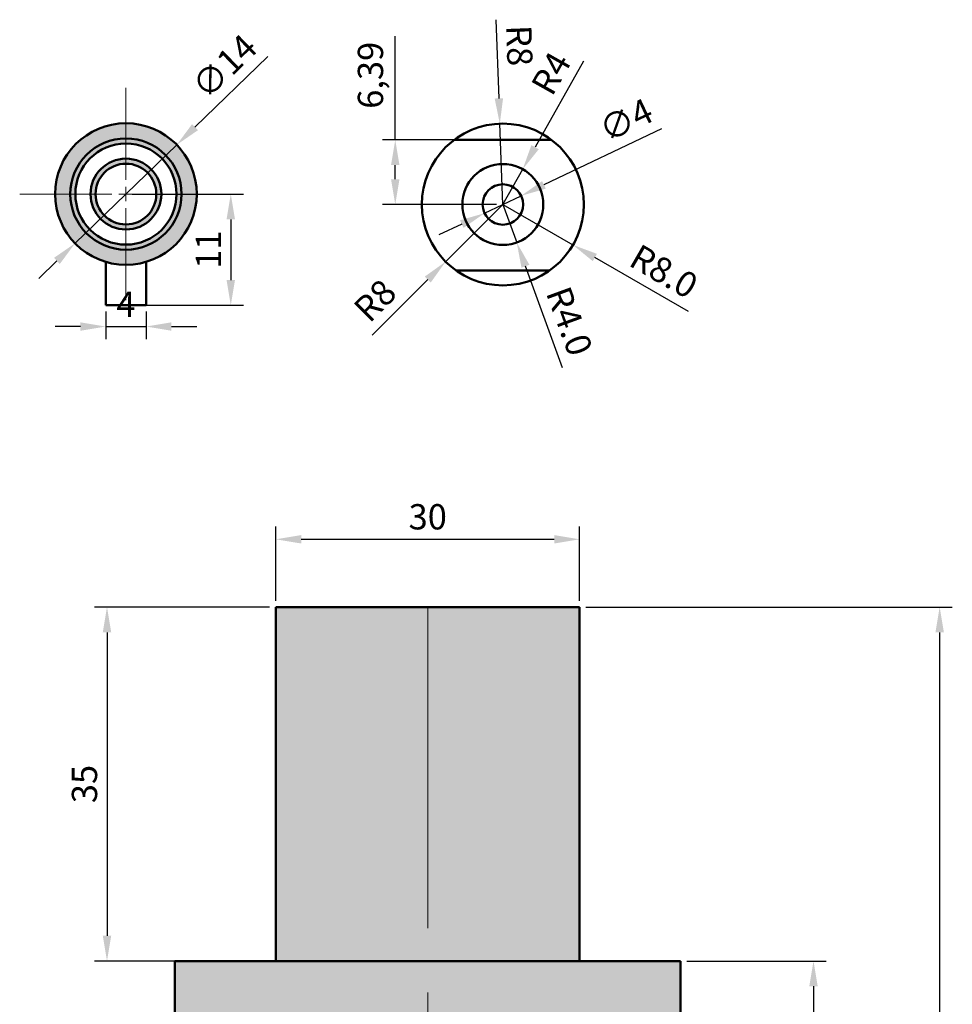
# Model space of a CAD drawing. Units: millimetres. Extents: x 1159 to 1466, y 1237 to 1440.
# Tile 3 of 6: x 1236 to 1329, y 1341 to 1438. Entities that reach past the tile are written whole.
import ezdxf

# ---------------------------------------------------------------- set-up
doc = ezdxf.new("R2010")
doc.units = ezdxf.units.MM
doc.linetypes.add('CENTER', pattern=[50.8, 31.75, -6.35, 6.35, -6.35])
for name, color, linetype, lineweight in [('M-CNTR', 1, 'CENTER', 18), ('M-DIMS', 2, 'Continuous', 25), ('M-HATC', 8, 'Continuous', 18), ('M-OUTL', 7, 'Continuous', 50)]:
    doc.layers.add(name, color=color, linetype=linetype, lineweight=lineweight)
doc.styles.get("Standard").update_dxf_attribs({"font": 'arial.ttf'})
doc.dimstyles.new('ISO-25', dxfattribs={"dimtxt": 2.5, "dimasz": 2.5, "dimexe": 1.25, "dimexo": 0.625, "dimtad": 1, "dimtxsty": 'Standard', "dimcen": 2.5, "dimadec": 0, "dimazin": 0, "dimtfac": 1, "dimtmove": 0, "dimatfit": 3, "dimfxl": 1, "dimarcsym": 0})

# ---------------------------------------------------------------- blocks, each defined once
blk = doc.blocks.new('*U1')
at = {"layer": 'M-CNTR', "color": 0, "transparency": 16777216}
for p, q in [((0, 1.4), (0, 10.5)), ((-10.5, 0), (-1.4, 0)), ((1.4, 0), (10.5, 0)), ((0, -10.5), (0, -1.4))]:
    blk.add_line(p, q, dxfattribs=at)
at = {"layer": 'M-CNTR', "color": 0, "linetype": 'Continuous', "transparency": 16777216}
for p, q in [((-0.7, 0), (0.7, 0)), ((0, -0.7), (0, 0.7))]:
    blk.add_line(p, q, dxfattribs=at)
blk = doc.blocks.new('*D3')
at = {"layer": 'Defpoints', "color": 0, "transparency": 16777216}
for p in [(1246.833, 1421.099), (1246.833, 1410.099), (1257.194, 1410.099)]:
    blk.add_point(p, dxfattribs=at)
at = {"layer": 'M-DIMS', "color": 0, "lineweight": -2, "transparency": 16777216}
for p, q in [((1247.458, 1421.099), (1258.444, 1421.099)), ((1257.194, 1418.599), (1257.194, 1412.599)), ((1247.458, 1410.099), (1258.444, 1410.099))]:
    blk.add_line(p, q, dxfattribs=at)
at = {"layer": 'M-DIMS', "color": 0, "transparency": 16777216}
for points in [[(1256.778, 1418.599), (1257.611, 1418.599), (1257.194, 1421.099)], [(1256.778, 1412.599), (1257.611, 1412.599), (1257.194, 1410.099)]]:
    blk.add_solid(points, dxfattribs=at)
at = {"layer": 'M-DIMS', "color": 0, "transparency": 16777216, "insert": (1255.314, 1415.599), "char_height": 2.5, "attachment_point": 5, "rotation": 90}
blk.add_mtext('11', dxfattribs=at)
blk = doc.blocks.new('*D4')
at = {"layer": 'Defpoints', "color": 0, "transparency": 16777216}
for p in [(1251.86, 1425.97), (1241.805, 1416.228)]:
    blk.add_point(p, dxfattribs=at)
at = {"layer": 'M-DIMS', "color": 0, "lineweight": -2, "transparency": 16777216}
for p, q in [((1260.867, 1434.697), (1253.656, 1427.71)), ((1241.805, 1416.228), (1251.86, 1425.97)), ((1240.01, 1414.489), (1238.215, 1412.749))]:
    blk.add_line(p, q, dxfattribs=at)
at = {"layer": 'M-DIMS', "color": 0, "transparency": 16777216}
for points in [[(1253.366, 1428.009), (1253.946, 1427.411), (1251.86, 1425.97)], [(1239.72, 1414.788), (1240.3, 1414.19), (1241.805, 1416.228)]]:
    blk.add_solid(points, dxfattribs=at)
at = {"layer": 'M-DIMS', "color": 0, "transparency": 16777216, "insert": (1256.787, 1433.489), "char_height": 2.5, "attachment_point": 5, "rotation": 44.0947}
blk.add_mtext('∅14', dxfattribs=at)
blk = doc.blocks.new('*D5')
at = {"layer": 'Defpoints', "color": 0, "transparency": 16777216}
for p in [(1273.452, 1426.462), (1284.087, 1426.462), (1284.087, 1420.067)]:
    blk.add_point(p, dxfattribs=at)
at = {"layer": 'M-DIMS', "color": 0, "lineweight": -2, "transparency": 16777216}
for p, q in [((1273.452, 1426.462), (1273.452, 1436.724)), ((1283.462, 1426.462), (1272.202, 1426.462)), ((1273.452, 1422.567), (1273.452, 1423.962)), ((1283.462, 1420.067), (1272.202, 1420.067))]:
    blk.add_line(p, q, dxfattribs=at)
at = {"layer": 'M-DIMS', "color": 0, "transparency": 16777216}
for points in [[(1273.036, 1423.962), (1273.869, 1423.962), (1273.452, 1426.462)], [(1273.036, 1422.567), (1273.869, 1422.567), (1273.452, 1420.067)]]:
    blk.add_solid(points, dxfattribs=at)
at = {"layer": 'M-DIMS', "color": 0, "transparency": 16777216, "insert": (1271.325, 1432.843), "char_height": 2.5, "attachment_point": 5, "rotation": 90}
blk.add_mtext('6,39', dxfattribs=at)
blk = doc.blocks.new('*D6')
at = {"layer": 'Defpoints', "color": 0, "transparency": 16777216}
for p in [(1285.892, 1420.928), (1282.282, 1419.206)]:
    blk.add_point(p, dxfattribs=at)
at = {"layer": 'M-DIMS', "color": 0, "lineweight": -2, "transparency": 16777216}
for p, q in [((1299.765, 1427.543), (1288.149, 1422.004)), ((1282.282, 1419.206), (1285.892, 1420.928)), ((1280.025, 1418.13), (1277.769, 1417.054))]:
    blk.add_line(p, q, dxfattribs=at)
at = {"layer": 'M-DIMS', "color": 0, "transparency": 16777216}
for points in [[(1287.969, 1422.38), (1288.328, 1421.628), (1285.892, 1420.928)], [(1279.846, 1418.506), (1280.204, 1417.754), (1282.282, 1419.206)]]:
    blk.add_solid(points, dxfattribs=at)
at = {"layer": 'M-DIMS', "color": 0, "transparency": 16777216, "insert": (1296.39, 1428.118), "char_height": 2.5, "attachment_point": 5, "rotation": 25.49518}
blk.add_mtext('∅4', dxfattribs=at)
blk = doc.blocks.new('*D7')
at = {"layer": 'Defpoints', "color": 0, "transparency": 16777216}
for p in [(1286.047, 1423.554), (1284.087, 1420.067)]:
    blk.add_point(p, dxfattribs=at)
at = {"layer": 'M-DIMS', "color": 0, "lineweight": -2, "transparency": 16777216}
for p, q in [((1292.064, 1434.254), (1287.273, 1425.733)), ((1284.087, 1420.067), (1286.047, 1423.554))]:
    blk.add_line(p, q, dxfattribs=at)
at = {"layer": 'M-DIMS', "color": 0, "transparency": 16777216}
blk.add_solid([(1286.909, 1425.937), (1287.636, 1425.529), (1286.047, 1423.554)], dxfattribs=at)
at = {"layer": 'M-DIMS', "color": 0, "transparency": 16777216, "insert": (1289.138, 1432.875), "char_height": 2.5, "attachment_point": 5, "rotation": 60.65232}
blk.add_mtext('R4', dxfattribs=at)
blk = doc.blocks.new('*D8')
at = {"layer": 'Defpoints', "color": 0, "transparency": 16777216}
for p in [(1283.788, 1428.061), (1284.087, 1420.067)]:
    blk.add_point(p, dxfattribs=at)
at = {"layer": 'M-DIMS', "color": 0, "lineweight": -2, "transparency": 16777216}
for p, q in [((1283.404, 1438.341), (1283.695, 1430.56)), ((1284.087, 1420.067), (1283.788, 1428.061))]:
    blk.add_line(p, q, dxfattribs=at)
at = {"layer": 'M-DIMS', "color": 0, "transparency": 16777216}
blk.add_solid([(1284.111, 1430.575), (1283.278, 1430.544), (1283.788, 1428.061)], dxfattribs=at)
at = {"layer": 'M-DIMS', "color": 0, "transparency": 16777216, "insert": (1285.403, 1435.77), "char_height": 2.5, "attachment_point": 5, "rotation": 272.1397}
blk.add_mtext('R8', dxfattribs=at)
blk = doc.blocks.new('*D17')
at = {"layer": 'Defpoints', "color": 0, "transparency": 16777216}
for p in [(1291.662, 1380.26), (1286.662, 1271.159), (1327.261, 1271.159)]:
    blk.add_point(p, dxfattribs=at)
at = {"layer": 'M-DIMS', "color": 0, "lineweight": -2, "transparency": 16777216}
for p, q in [((1292.287, 1380.26), (1328.511, 1380.26)), ((1327.261, 1377.76), (1327.261, 1273.659)), ((1287.287, 1271.159), (1328.511, 1271.159))]:
    blk.add_line(p, q, dxfattribs=at)
at = {"layer": 'M-DIMS', "color": 0, "transparency": 16777216}
for points in [[(1326.844, 1377.76), (1327.678, 1377.76), (1327.261, 1380.26)], [(1326.844, 1273.659), (1327.678, 1273.659), (1327.261, 1271.159)]]:
    blk.add_solid(points, dxfattribs=at)
at = {"layer": 'M-DIMS', "color": 0, "transparency": 16777216, "insert": (1325.134, 1325.71), "char_height": 2.5, "attachment_point": 5, "rotation": 90}
blk.add_mtext('109,1', dxfattribs=at)
blk = doc.blocks.new('*D18')
at = {"layer": 'Defpoints', "color": 0, "transparency": 16777216}
for p in [(1301.662, 1345.26), (1300.162, 1322.76), (1314.79, 1322.76)]:
    blk.add_point(p, dxfattribs=at)
at = {"layer": 'M-DIMS', "color": 0, "lineweight": -2, "transparency": 16777216}
for p, q in [((1302.287, 1345.26), (1316.04, 1345.26)), ((1314.79, 1342.76), (1314.79, 1325.26)), ((1300.787, 1322.76), (1316.04, 1322.76))]:
    blk.add_line(p, q, dxfattribs=at)
at = {"layer": 'M-DIMS', "color": 0, "transparency": 16777216}
for points in [[(1314.373, 1342.76), (1315.207, 1342.76), (1314.79, 1345.26)], [(1314.373, 1325.26), (1315.207, 1325.26), (1314.79, 1322.76)]]:
    blk.add_solid(points, dxfattribs=at)
at = {"layer": 'M-DIMS', "color": 0, "transparency": 16777216, "insert": (1312.663, 1334.01), "char_height": 2.5, "attachment_point": 5, "rotation": 90}
blk.add_mtext('22,5', dxfattribs=at)
blk = doc.blocks.new('*D29')
at = {"layer": 'Defpoints', "color": 0, "transparency": 16777216}
for p in [(1291.662, 1386.96), (1261.662, 1380.26), (1291.662, 1380.26)]:
    blk.add_point(p, dxfattribs=at)
at = {"layer": 'M-DIMS', "color": 0, "lineweight": -2, "transparency": 16777216}
for p, q in [((1261.662, 1380.885), (1261.662, 1388.21)), ((1291.662, 1380.885), (1291.662, 1388.21)), ((1264.162, 1386.96), (1289.162, 1386.96))]:
    blk.add_line(p, q, dxfattribs=at)
at = {"layer": 'M-DIMS', "color": 0, "transparency": 16777216}
for points in [[(1264.162, 1387.377), (1264.162, 1386.544), (1261.662, 1386.96)], [(1289.162, 1387.377), (1289.162, 1386.544), (1291.662, 1386.96)]]:
    blk.add_solid(points, dxfattribs=at)
at = {"layer": 'M-DIMS', "color": 0, "transparency": 16777216, "insert": (1276.662, 1388.863), "char_height": 2.5, "attachment_point": 5}
blk.add_mtext('30', dxfattribs=at)
blk = doc.blocks.new('*D33')
at = {"layer": 'Defpoints', "color": 0, "transparency": 16777216}
for p in [(1261.662, 1380.26), (1244.962, 1345.26), (1261.662, 1345.26)]:
    blk.add_point(p, dxfattribs=at)
at = {"layer": 'M-DIMS', "color": 0, "lineweight": -2, "transparency": 16777216}
for p, q in [((1261.037, 1380.26), (1243.712, 1380.26)), ((1244.962, 1377.76), (1244.962, 1347.76)), ((1261.037, 1345.26), (1243.712, 1345.26))]:
    blk.add_line(p, q, dxfattribs=at)
at = {"layer": 'M-DIMS', "color": 0, "transparency": 16777216}
for points in [[(1244.545, 1377.76), (1245.378, 1377.76), (1244.962, 1380.26)], [(1244.545, 1347.76), (1245.378, 1347.76), (1244.962, 1345.26)]]:
    blk.add_solid(points, dxfattribs=at)
at = {"layer": 'M-DIMS', "color": 0, "transparency": 16777216, "insert": (1243.059, 1362.76), "char_height": 2.5, "attachment_point": 5, "rotation": 90}
blk.add_mtext('35', dxfattribs=at)
blk = doc.blocks.new('*D41')
at = {"layer": 'Defpoints', "color": 0, "transparency": 16777216}
for p in [(1244.833, 1410.099), (1248.833, 1410.099), (1248.833, 1407.999)]:
    blk.add_point(p, dxfattribs=at)
at = {"layer": 'M-DIMS', "color": 0, "lineweight": -2, "transparency": 16777216}
for p, q in [((1244.833, 1409.474), (1244.833, 1406.749)), ((1248.833, 1409.474), (1248.833, 1406.749)), ((1242.333, 1407.999), (1239.833, 1407.999)), ((1244.833, 1407.999), (1248.833, 1407.999)), ((1251.333, 1407.999), (1253.833, 1407.999))]:
    blk.add_line(p, q, dxfattribs=at)
at = {"layer": 'M-DIMS', "color": 0, "transparency": 16777216}
for points in [[(1242.333, 1408.416), (1242.333, 1407.583), (1244.833, 1407.999)], [(1251.333, 1408.416), (1251.333, 1407.583), (1248.833, 1407.999)]]:
    blk.add_solid(points, dxfattribs=at)
at = {"layer": 'M-DIMS', "color": 0, "transparency": 16777216, "insert": (1246.833, 1409.874), "char_height": 2.5, "attachment_point": 5}
blk.add_mtext('4', dxfattribs=at)
blk = doc.blocks.new('*D53')
at = {"layer": 'Defpoints', "color": 0, "transparency": 16777216}
for p in [(1284.087, 1420.067), (1278.43, 1414.41)]:
    blk.add_point(p, dxfattribs=at)
at = {"layer": 'M-DIMS', "color": 0, "lineweight": -2, "transparency": 16777216}
for p, q in [((1284.087, 1420.067), (1278.43, 1414.41)), ((1271.156, 1407.136), (1276.662, 1412.642))]:
    blk.add_line(p, q, dxfattribs=at)
at = {"layer": 'M-DIMS', "color": 0, "transparency": 16777216}
blk.add_solid([(1276.368, 1412.937), (1276.957, 1412.348), (1278.43, 1414.41)], dxfattribs=at)
at = {"layer": 'M-DIMS', "color": 0, "transparency": 16777216, "insert": (1271.681, 1410.35), "char_height": 2.5, "attachment_point": 5, "rotation": 45.00022}
blk.add_mtext('R8', dxfattribs=at)
blk = doc.blocks.new('*D92')
at = {"layer": 'Defpoints', "color": 0, "transparency": 16777216}
for p in [(1284.087, 1420.067), (1291.018, 1416.071)]:
    blk.add_point(p, dxfattribs=at)
at = {"layer": 'M-DIMS', "color": 0, "lineweight": -2, "transparency": 16777216}
for p, q in [((1284.087, 1420.067), (1291.018, 1416.071)), ((1302.441, 1409.486), (1293.184, 1414.823))]:
    blk.add_line(p, q, dxfattribs=at)
at = {"layer": 'M-DIMS', "color": 0, "transparency": 16777216}
blk.add_solid([(1293.392, 1415.184), (1292.975, 1414.462), (1291.018, 1416.071)], dxfattribs=at)
at = {"layer": 'M-DIMS', "color": 0, "transparency": 16777216, "insert": (1299.845, 1413.177), "char_height": 2.5, "attachment_point": 5, "rotation": 330.03652}
blk.add_mtext('R8.0', dxfattribs=at)
blk = doc.blocks.new('*D93')
at = {"layer": 'Defpoints', "color": 0, "transparency": 16777216}
for p in [(1284.087, 1420.067), (1285.46, 1416.31)]:
    blk.add_point(p, dxfattribs=at)
at = {"layer": 'M-DIMS', "color": 0, "lineweight": -2, "transparency": 16777216}
for p, q in [((1284.087, 1420.067), (1285.46, 1416.31)), ((1289.986, 1403.926), (1286.318, 1413.962))]:
    blk.add_line(p, q, dxfattribs=at)
at = {"layer": 'M-DIMS', "color": 0, "transparency": 16777216}
blk.add_solid([(1286.71, 1414.105), (1285.927, 1413.819), (1285.46, 1416.31)], dxfattribs=at)
at = {"layer": 'M-DIMS', "color": 0, "transparency": 16777216, "insert": (1290.367, 1408.422), "char_height": 2.5, "attachment_point": 5, "rotation": 290.07659}
blk.add_mtext('R4.0', dxfattribs=at)

msp = doc.modelspace()

# ---------------------------------------------------------------- hatches: boundary and pattern name
at = {"layer": 'M-HATC'}
h = msp.add_hatch(color=256, dxfattribs=at)
h.set_gradient(color1=(19, 103, 52))
h.paths.add_polyline_path([(1239.8328, 1421.0994), (1241.3328, 1421.0994, -0.4142136), (1246.8328, 1426.5994), (1246.8328, 1428.0994, 0.4142136)])
h.paths.add_polyline_path([(1246.8328, 1428.0994), (1246.8328, 1426.5994, -0.4142136), (1252.3328, 1421.0994), (1253.8328, 1421.0994, 0.4142136)])
h.paths.add_polyline_path([(1246.8328, 1415.5994), (1246.8328, 1414.0994, 0.4142136), (1253.8328, 1421.0994), (1252.3328, 1421.0994, -0.4142136)])
h.paths.add_polyline_path([(1246.8328, 1414.0994), (1246.8328, 1415.5994, -0.4142136), (1241.3328, 1421.0994), (1239.8328, 1421.0994, 0.4142136)])
h = msp.add_hatch(color=256, dxfattribs=at)
h.set_gradient(color1=(205, 32, 39))
h.paths.add_polyline_path([(1246.8328, 1426.0994), (1246.8328, 1426.5994, 0.4142136), (1241.3328, 1421.0994), (1241.8328, 1421.0994, -0.4142136)])
h.paths.add_polyline_path([(1251.8328, 1421.0994), (1252.3328, 1421.0994, 0.4142136), (1246.8328, 1426.5994), (1246.8328, 1426.0994, -0.4142136)])
h.paths.add_polyline_path([(1246.8328, 1416.0994), (1246.8328, 1415.5994, 0.4142136), (1252.3328, 1421.0994), (1251.8328, 1421.0994, -0.4142136)])
h.paths.add_polyline_path([(1241.8328, 1421.0994), (1241.3328, 1421.0994, 0.4142136), (1246.8328, 1415.5994), (1246.8328, 1416.0994, -0.4142136)])
h = msp.add_hatch(color=256, dxfattribs=at)
h.set_gradient(color2=(0, 0, 255))
h.paths.add_polyline_path([(1246.8328, 1424.0994), (1246.8328, 1424.5994, 0.4142136), (1243.3328, 1421.0994), (1243.8328, 1421.0994, -0.4142136)])
h.paths.add_polyline_path([(1249.8328, 1421.0994), (1250.3328, 1421.0994, 0.4142136), (1246.8328, 1424.5994), (1246.8328, 1424.0994, -0.4142136)])
h.paths.add_polyline_path([(1250.3328, 1421.0994), (1249.8328, 1421.0994, -0.4142136), (1246.8328, 1418.0994), (1246.8328, 1417.5994, 0.4142136)])
h.paths.add_polyline_path([(1243.8328, 1421.0994), (1243.3328, 1421.0994, 0.4142136), (1246.8328, 1417.5994), (1246.8328, 1418.0994, -0.4142136)])
h = msp.add_hatch(color=256, dxfattribs=at)
h.set_gradient(color1=(100, 33, 101))
h.paths.add_polyline_path([(1276.6615, 1380.2603), (1261.6615, 1380.2603), (1261.6615, 1345.2603), (1276.6615, 1345.2603)])
h.paths.add_polyline_path([(1291.6615, 1380.2603), (1276.6615, 1380.2603), (1276.6615, 1345.2603), (1291.6615, 1345.2603)])
h = msp.add_hatch(color=256, dxfattribs=at)
h.set_gradient(color1=(237, 31, 36), color2=(248, 215, 49))
h.paths.add_polyline_path([(1276.6615, 1345.2603), (1261.6615, 1345.2603), (1251.6615, 1345.2603), (1251.6615, 1322.7603), (1254.6615, 1322.7603), (1276.6615, 1322.7603)])
h.paths.add_polyline_path([(1301.6615, 1345.2603), (1291.6615, 1345.2603), (1276.6615, 1345.2603), (1276.6615, 1322.7603), (1298.6615, 1322.7603), (1301.6615, 1322.7603)])

# ---------------------------------------------------------------- linework, layer by layer
at = {"layer": 'M-CNTR'}
msp.add_line((1276.6615, 1380.2603), (1276.6615, 1271.159), dxfattribs=at)
at = {"layer": 'M-OUTL'}
for p, q in [((1279.2799, 1426.4617), (1288.8939, 1426.4617)), ((1244.8328, 1414.3912), (1244.8328, 1410.0994)), ((1248.8328, 1410.0994), (1248.8328, 1414.3912)), ((1288.6931, 1413.5261), (1279.4807, 1413.5261)), ((1246.8328, 1410.0994), (1244.8328, 1410.0994)), ((1246.8328, 1410.0994), (1248.8328, 1410.0994)), ((1261.6615, 1380.2603), (1291.6615, 1380.2603)), ((1261.6615, 1345.2603), (1261.6615, 1380.2603)), ((1291.6615, 1380.2603), (1291.6615, 1345.2603)), ((1261.6615, 1345.2603), (1251.6615, 1345.2603)), ((1251.6615, 1345.2603), (1251.6615, 1322.7603)), ((1291.6615, 1345.2603), (1261.6615, 1345.2603)), ((1301.6615, 1345.2603), (1291.6615, 1345.2603)), ((1301.6615, 1322.7603), (1301.6615, 1345.2603))]:
    msp.add_line(p, q, dxfattribs=at)
for centre, radius in [((1246.8328, 1421.0994), 7), ((1284.0869, 1420.0669), 8), ((1246.8328, 1421.0994), 5.5), ((1246.8328, 1421.0994), 5), ((1246.8328, 1421.0994), 3.5), ((1246.8328, 1421.0994), 3), ((1284.0869, 1420.0669), 4), ((1284.0869, 1420.0669), 2)]:
    msp.add_circle(centre, radius, dxfattribs=at)

# ---------------------------------------------------------------- block references
at = {"layer": 'M-CNTR'}
msp.add_blockref('*U1', (1246.8328, 1421.0994), dxfattribs=at)

# ---------------------------------------------------------------- dimensions: what is measured, and where the dimension line sits
at = {"layer": 'M-DIMS'}
for mpoint, override, picture, middle in [((1283.7882, 1428.0614), {"dimclrd": 0, "dimclre": 0, "dimclrt": 0}, '*D8', (1285.4029, 1435.7703)), ((1278.4301, 1414.4101), {"dimdec": 0, "dimlfac": 1, "dimrnd": 0, "dimzin": 0, "dimdsep": 46, "dimlunit": 2}, '*D53', (1271.681, 1410.35)), ((1291.0176, 1416.0714), {"dimdec": 1, "dimlfac": 1, "dimrnd": 0, "dimzin": 0, "dimdsep": 46, "dimlunit": 2}, '*D92', (1299.8448, 1413.1773)), ((1285.46, 1416.31), {"dimdec": 1, "dimlfac": 1, "dimrnd": 0, "dimzin": 0, "dimdsep": 46, "dimlunit": 2}, '*D93', (1290.3672, 1408.4225))]:
    dim = msp.add_radius_dim(center=(1284.0869, 1420.0669), mpoint=mpoint, dimstyle='ISO-25', override=override, dxfattribs=at)
    dim.commit()
    dim.dimension.update_dxf_attribs({"geometry": picture, "text_midpoint": middle})
dim = msp.add_diameter_dim_2p(p1=(1241.8055, 1416.2284), p2=(1251.8602, 1425.9703), dimstyle='ISO-25', override={"dimclrd": 0, "dimclre": 0, "dimclrt": 0}, dxfattribs=at)
dim.commit()
dim.dimension.update_dxf_attribs({"geometry": '*D4', "text_midpoint": (1256.7873, 1433.489)})
for base, p1, p2, override, picture, middle in [((1273.4525, 1426.4617), (1284.0869, 1420.0669), (1284.0869, 1426.4617), {"dimclrd": 0, "dimclre": 0, "dimclrt": 0}, '*D5', (1271.3251, 1432.843)), ((1257.1943, 1410.0994), (1246.8328, 1421.0994), (1246.8328, 1410.0994), {"dimclrd": 0, "dimclre": 0, "dimclrt": 0}, '*D3', (1255.3142, 1415.5994)), ((1244.9615, 1345.2603), (1261.6615, 1380.2603), (1261.6615, 1345.2603), {"dimdec": 0, "dimlfac": 1, "dimrnd": 0, "dimzin": 0, "dimdsep": 46, "dimlunit": 2}, '*D33', (1243.0593, 1362.7603)), ((1327.2609, 1271.159), (1291.6615, 1380.2603), (1286.6615, 1271.159), {"dimclrd": 0, "dimclre": 0, "dimclrt": 0}, '*D17', (1325.1335, 1325.7096)), ((1314.79, 1322.7603), (1301.6615, 1345.2603), (1300.1615, 1322.7603), {"dimclrd": 0, "dimclre": 0, "dimclrt": 0}, '*D18', (1312.6626, 1334.0103))]:
    dim = msp.add_linear_dim(base=base, p1=p1, p2=p2, angle=90, dimstyle='ISO-25', override=override, dxfattribs=at)
    dim.commit()
    dim.dimension.update_dxf_attribs({"geometry": picture, "text_midpoint": middle})
dim = msp.add_radius_dim(center=(1284.0869, 1420.0669), mpoint=(1286.0473, 1423.5536), dimstyle='ISO-25', override={"dimclrd": 0, "dimclre": 0, "dimclrt": 0}, dxfattribs=at)
dim.commit()
dim.dimension.update_dxf_attribs({"geometry": '*D7', "text_midpoint": (1290.772, 1431.9565), "dimtype": 164})
dim = msp.add_diameter_dim_2p(p1=(1282.2817, 1419.2061), p2=(1285.8921, 1420.9278), dimstyle='ISO-25', override={"dimclrd": 0, "dimclre": 0, "dimclrt": 0}, dxfattribs=at)
dim.commit()
dim.dimension.update_dxf_attribs({"geometry": '*D6', "text_midpoint": (1297.2383, 1426.3385), "dimtype": 163})
for base, p1, p2, picture, middle in [((1248.8328, 1407.9994), (1244.8328, 1410.0994), (1248.8328, 1410.0994), '*D41', (1246.8328, 1409.8744)), ((1291.6615, 1386.9603), (1261.6615, 1380.2603), (1291.6615, 1380.2603), '*D29', (1276.6615, 1388.8625))]:
    dim = msp.add_linear_dim(base=base, p1=p1, p2=p2, dimstyle='ISO-25', override={"dimdec": 0, "dimlfac": 1, "dimrnd": 0, "dimzin": 0, "dimdsep": 46, "dimlunit": 2}, dxfattribs=at)
    dim.commit()
    dim.dimension.update_dxf_attribs({"geometry": picture, "text_midpoint": middle})

doc.saveas('drawing.dxf')
